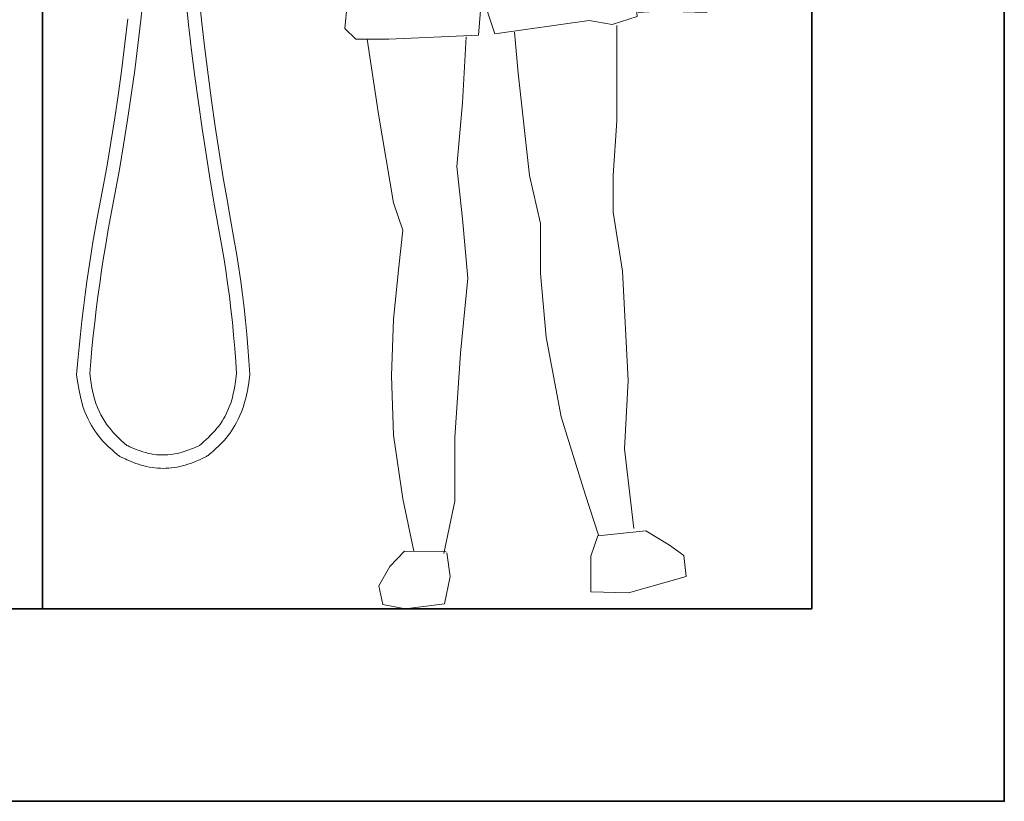
# Model space of a CAD drawing. Units: inches. Extents: x 64 to 1167, y 117 to 939.
# Tile 38 of 56: x 1121 to 1167, y 428 to 464. Entities that reach past the tile are written whole.
import ezdxf

# ---------------------------------------------------------------- set-up
doc = ezdxf.new("R2010")
doc.units = ezdxf.units.IN
doc.header["$MEASUREMENT"] = 0
for name, color, linetype, lineweight in [('A-ENTG', 8, 'Continuous', 18), ('A-FLOR-FIXT', 8, 'Continuous', 18), ('A-SECT', 7, 'Continuous', 35)]:
    doc.layers.add(name, color=color, linetype=linetype, lineweight=lineweight)

# ---------------------------------------------------------------- blocks, each defined once
blk = doc.blocks.new('A$C43851DCA')
at = {"linetype": 'ByBlock'}
for p, q in [((0.009394, 0.066918), (0.008245, 0.066783)), ((0.010881, 0.066467), (0.009394, 0.066918)), ((0.008245, 0.066783), (0.007206, 0.066287)), ((0.011698, 0.06601), (0.010881, 0.066467)), ((0.007206, 0.066287), (0.0065, 0.065469)), ((0.012995, 0.064742), (0.011698, 0.06601)), ((0.0065, 0.065469), (0.005873, 0.063886)), ((0.013812, 0.064066), (0.012995, 0.064742)), ((0.014181, 0.063564), (0.013812, 0.064066)), ((0.005873, 0.063886), (0.005683, 0.062753)), ((0.013627, 0.063023), (0.014107, 0.063203)), ((0.014107, 0.063203), (0.014181, 0.063564)), ((0.005683, 0.062753), (0.005535, 0.061845)), ((0.009658, 0.062341), (0.010064, 0.062753)), ((0.010064, 0.062753), (0.01047, 0.062843)), ((0.01047, 0.062843), (0.010807, 0.062708)), ((0.010807, 0.062708), (0.010844, 0.062566)), ((0.012215, 0.062115), (0.012995, 0.062798)), ((0.012995, 0.062798), (0.013627, 0.063023)), ((0.01359, 0.062978), (0.013179, 0.061298)), ((0.009658, 0.061755), (0.009658, 0.062341)), ((0.005535, 0.061845), (0.005461, 0.060802)), ((0.009953, 0.061163), (0.009658, 0.061755)), ((0.011882, 0.061343), (0.012215, 0.062115)), ((0.009732, 0.061343), (0.009173, 0.060757)), ((0.011846, 0.060712), (0.011882, 0.061343)), ((0.013179, 0.061298), (0.013069, 0.060757)), ((0.010322, 0.060757), (0.009953, 0.061163)), ((0.005461, 0.060802), (0.005683, 0.060397)), ((0.005683, 0.060397), (0.00602, 0.060165)), ((0.009173, 0.060757), (0.008393, 0.059804)), ((0.010543, 0.06021), (0.010322, 0.060757)), ((0.013069, 0.060757), (0.013253, 0.060442)), ((0.013253, 0.060442), (0.013364, 0.06003)), ((0.00602, 0.060165), (0.0065, 0.059624)), ((0.013364, 0.06003), (0.013179, 0.059624)), ((0.0065, 0.059624), (0.006721, 0.058807)), ((0.007728, 0.059534), (0.006911, 0.059444)), ((0.008393, 0.059804), (0.007728, 0.059534)), ((0.013179, 0.059624), (0.012552, 0.058897)), ((0.006721, 0.058807), (0.006948, 0.057674)), ((0.010844, 0.057764), (0.01047, 0.058897)), ((0.012552, 0.058897), (0.012215, 0.058446)), ((0.012215, 0.058446), (0.012067, 0.057905)), ((0.006948, 0.057674), (0.006948, 0.057313)), ((0.010733, 0.056772), (0.010623, 0.057809)), ((0.01125, 0.057538), (0.010844, 0.057764)), ((0.012067, 0.057905), (0.011882, 0.057538)), ((0.005999, 0.057487), (0.00523, 0.056785)), ((0.00689, 0.057326), (0.005999, 0.057487)), ((0.009953, 0.057017), (0.00689, 0.057326)), ((0.011882, 0.057538), (0.01125, 0.057538)), ((0.00523, 0.056785), (0.004086, 0.055614)), ((0.011355, 0.05647), (0.009953, 0.057017)), ((0.013269, 0.055614), (0.011355, 0.05647)), ((0.004086, 0.055614), (0.00185, 0.054133)), ((0.01397, 0.054912), (0.013269, 0.055614)), ((0.014223, 0.052266), (0.01397, 0.054912)), ((0.00185, 0.054133), (0.000828, 0.053199)), ((0.000828, 0.053199), (0.000511, 0.050476)), ((0.014292, 0.049929), (0.014223, 0.052266)), ((0.010654, 0.051642), (0.01097, 0.051172)), ((0.01097, 0.051172), (0.010781, 0.048294)), ((0.000511, 0.050476), (0.00019, 0.04915)), ((0.01416, 0.047122), (0.014292, 0.049929)), ((0.00019, 0.04915), (0, 0.047747)), ((0.002615, 0.048758), (0.002235, 0.047438)), ((0.010781, 0.048294), (0.011102, 0.046035)), ((0, 0.047747), (0.000258, 0.045726)), ((0.002235, 0.047438), (0.002552, 0.045256)), ((0.012378, 0.046582), (0.01378, 0.047045)), ((0.01378, 0.047045), (0.01416, 0.047122)), ((0.011102, 0.046035), (0.012378, 0.046582)), ((0.01397, 0.046891), (0.01416, 0.04541)), ((0.011545, 0.046112), (0.011419, 0.044863)), ((0.000258, 0.045726), (0.000448, 0.043775)), ((0.002552, 0.045256), (0.002936, 0.043151)), ((0.01416, 0.04541), (0.015119, 0.044863)), ((0.011419, 0.044863), (0.011419, 0.043775)), ((0.015119, 0.044863), (0.016522, 0.044084)), ((0.000448, 0.043775), (0.000638, 0.042449)), ((0.011419, 0.043775), (0.012056, 0.043228)), ((0.016522, 0.044084), (0.017349, 0.043389)), ((0.017349, 0.043389), (0.017924, 0.042217)), ((0.002936, 0.043151), (0.003063, 0.041284)), ((0.012056, 0.043228), (0.013522, 0.042842)), ((0.000638, 0.042449), (0.001276, 0.042217)), ((0.013522, 0.042842), (0.015309, 0.042449)), ((0.015309, 0.042449), (0.016458, 0.041515)), ((0.001276, 0.042217), (0.002936, 0.041438)), ((0.014929, 0.039726), (0.015119, 0.042294)), ((0.017924, 0.042217), (0.018435, 0.041129)), ((0.016458, 0.041515), (0.01697, 0.040736)), ((0.003063, 0.041284), (0.003253, 0.040035)), ((0.020871, 0.040711), (0.016163, 0.04046)), ((0.022052, 0.028454), (0.020871, 0.040711)), ((0.015135, 0.040151), (0.019901, 0.040209)), ((0.019901, 0.040209), (0.021335, 0.028512)), ((0.003253, 0.040035), (0.003379, 0.037775)), ((0.01397, 0.039494), (0.014929, 0.039726)), ((0.016316, 0.037395), (0.015082, 0.039713)), ((0.01174, 0.03887), (0.012441, 0.039333)), ((0.012441, 0.039333), (0.01397, 0.039494)), ((0.011034, 0.038631), (0.01174, 0.03887)), ((0.003891, 0.037074), (0.011034, 0.038631)), ((0.003379, 0.037775), (0.003891, 0.037074)), ((0.016775, 0.035709), (0.016316, 0.037395)), ((0.003917, 0.037022), (0.003253, 0.035458)), ((0.016927, 0.034453), (0.016775, 0.035709)), ((0.003253, 0.035458), (0.003147, 0.03352)), ((0.016775, 0.033018), (0.016927, 0.034453)), ((0.003147, 0.03352), (0.003147, 0.03164)), ((0.008424, 0.033456), (0.008377, 0.032329)), ((0.016674, 0.030707), (0.016775, 0.033018)), ((0.008377, 0.032329), (0.008683, 0.030765)), ((0.003147, 0.03164), (0.003305, 0.029954)), ((0.008683, 0.030765), (0.0095, 0.029452)), ((0.016927, 0.027701), (0.016674, 0.030707)), ((0.003305, 0.029954), (0.003353, 0.028267)), ((0.0095, 0.029452), (0.009964, 0.027829)), ((0.0095, 0.026825), (0.009658, 0.028705)), ((0.003353, 0.028267), (0.003253, 0.02714)), ((0.021335, 0.028512), (0.020154, 0.027887)), ((0.020565, 0.028138), (0.022052, 0.028454)), ((0.009964, 0.027829), (0.010269, 0.026889)), ((0.015752, 0.027327), (0.016927, 0.027701)), ((0.018003, 0.027952), (0.01698, 0.027887)), ((0.020154, 0.027887), (0.018003, 0.027952)), ((0.010269, 0.026889), (0.014676, 0.027514)), ((0.014676, 0.027514), (0.015752, 0.027327)), ((0.015984, 0.022814), (0.015984, 0.027282)), ((0.003253, 0.02714), (0.003764, 0.026638)), ((0.005303, 0.026638), (0.0095, 0.026825)), ((0.008751, 0.023664), (0.008925, 0.026748)), ((0.011192, 0.02696), (0.011366, 0.025048)), ((0.003764, 0.026638), (0.005303, 0.026638)), ((0.004302, 0.026645), (0.004829, 0.02313)), ((0.011366, 0.025048), (0.011888, 0.020259)), ((0.008487, 0.020684), (0.008751, 0.023664)), ((0.004829, 0.02313), (0.005525, 0.018978)), ((0.01581, 0.020259), (0.015984, 0.022814)), ((0.008751, 0.018237), (0.008487, 0.020684)), ((0.011888, 0.020259), (0.01241, 0.018025)), ((0.01581, 0.018553), (0.01581, 0.020259)), ((0.005525, 0.018978), (0.005962, 0.017703)), ((0.016247, 0.015785), (0.01581, 0.018553)), ((0.009009, 0.015469), (0.008751, 0.018237)), ((0.01241, 0.018025), (0.01241, 0.015682)), ((0.005962, 0.017703), (0.005783, 0.015997)), ((0.005783, 0.015997), (0.005525, 0.013551)), ((0.01241, 0.015682), (0.012673, 0.012701)), ((0.016506, 0.01068), (0.016247, 0.015785)), ((0.008661, 0.011954), (0.009009, 0.015469)), ((0.005525, 0.013551), (0.005435, 0.010892)), ((0.012673, 0.012701), (0.013369, 0.008974)), ((0.008403, 0.008015), (0.008661, 0.011954)), ((0.005435, 0.010892), (0.005525, 0.008124)), ((0.016332, 0.007487), (0.016506, 0.01068)), ((0.013369, 0.008974), (0.014502, 0.005356)), ((0.005525, 0.008124), (0.005962, 0.005144)), ((0.008403, 0.005034), (0.008403, 0.008015)), ((0.016769, 0.003759), (0.016332, 0.007487)), ((0.005962, 0.005144), (0.006484, 0.002697)), ((0.014502, 0.005356), (0.015114, 0.003438)), ((0.007876, 0.002588), (0.008403, 0.005034)), ((0.015093, 0.003412), (0.014766, 0.002459)), ((0.017333, 0.003644), (0.015093, 0.003412)), ((0.018435, 0.002974), (0.017333, 0.003644)), ((0.019115, 0.002498), (0.018435, 0.002974)), ((0.006036, 0.002697), (0.005356, 0.001983)), ((0.007987, 0.002659), (0.006036, 0.002697)), ((0.008182, 0.001506), (0.008018, 0.002614)), ((0.014766, 0.002459), (0.014766, 0.000792)), ((0.019215, 0.001506), (0.019115, 0.002498)), ((0.005356, 0.001983), (0.004839, 0.001069)), ((0.007918, 0.000238), (0.008182, 0.001506)), ((0.016522, 0.000753), (0.019215, 0.001506)), ((0.004839, 0.001069), (0.005034, 0.0002)), ((0.014766, 0.000792), (0.016522, 0.000753)), ((0.005034, 0.0002), (0.006073, 0)), ((0.006073, 0), (0.007918, 0.000238))]:
    blk.add_line(p, q, dxfattribs=at)

msp = doc.modelspace()

# ---------------------------------------------------------------- linework, layer by layer
at = {"layer": 'A-FLOR-FIXT'}
for p, q in [((1126.404, 464.201), (1126.528, 465.37)), ((1128.515, 465.221), (1128.645, 464.002)), ((1129.26, 464.072), (1129.136, 465.244)), ((1125.667, 463.108), (1125.802, 464.269)), ((1126.268, 463.034), (1126.404, 464.201)), ((1128.645, 464.002), (1128.786, 462.785)), ((1129.4, 462.861), (1129.26, 464.072)), ((1125.519, 461.949), (1125.667, 463.108)), ((1126.12, 461.868), (1126.268, 463.034)), ((1128.786, 462.785), (1128.938, 461.57)), ((1129.552, 461.651), (1129.4, 462.861)), ((1125.36, 460.791), (1125.519, 461.949)), ((1125.96, 460.704), (1126.12, 461.868)), ((1128.938, 461.57), (1129.101, 460.356)), ((1129.714, 460.443), (1129.552, 461.651)), ((1125.189, 459.636), (1125.36, 460.791)), ((1125.788, 459.542), (1125.96, 460.704)), ((1129.101, 460.356), (1129.275, 459.144)), ((1129.887, 459.237), (1129.714, 460.443)), ((1125.006, 458.483), (1125.189, 459.636)), ((1125.604, 458.383), (1125.788, 459.542)), ((1129.275, 459.144), (1129.46, 457.935)), ((1130.071, 458.033), (1129.887, 459.237)), ((1124.811, 457.332), (1125.006, 458.483)), ((1125.407, 457.226), (1125.604, 458.383)), ((1130.266, 456.831), (1130.071, 458.033)), ((1129.46, 457.935), (1129.656, 456.727)), ((1124.603, 456.184), (1124.811, 457.332)), ((1125.199, 456.072), (1125.407, 457.226)), ((1129.656, 456.727), (1129.863, 455.521)), ((1130.472, 455.631), (1130.266, 456.831)), ((1124.384, 455.037), (1124.603, 456.184)), ((1124.98, 454.924), (1125.199, 456.072)), ((1130.188, 453.716), (1129.863, 455.521)), ((1130.558, 455.155), (1130.472, 455.631)), ((1124.273, 454.428), (1124.384, 455.034)), ((1124.87, 454.32), (1124.98, 454.924)), ((1130.797, 453.824), (1130.558, 455.155)), ((1124.168, 453.819), (1124.273, 454.428)), ((1124.765, 453.717), (1124.87, 454.32)), ((1130.9, 453.214), (1130.797, 453.824)), ((1124.068, 453.209), (1124.168, 453.819)), ((1124.666, 453.112), (1124.765, 453.717)), ((1130.188, 453.716), (1130.289, 453.113)), ((1123.973, 452.597), (1124.068, 453.209)), ((1124.572, 452.506), (1124.666, 453.112)), ((1130.289, 453.113), (1130.383, 452.508)), ((1130.995, 452.602), (1130.9, 453.214)), ((1123.884, 451.985), (1123.973, 452.597)), ((1124.484, 451.899), (1124.572, 452.506)), ((1130.383, 452.508), (1130.471, 451.903)), ((1131.084, 451.989), (1130.995, 452.602)), ((1123.8, 451.372), (1123.884, 451.985)), ((1131.165, 451.375), (1131.084, 451.989)), ((1124.401, 451.291), (1124.484, 451.899)), ((1130.471, 451.903), (1130.552, 451.296)), ((1123.721, 450.758), (1123.8, 451.372)), ((1124.323, 450.683), (1124.401, 451.291)), ((1130.552, 451.296), (1130.625, 450.688)), ((1131.24, 450.76), (1131.165, 451.375)), ((1123.648, 450.143), (1123.721, 450.758)), ((1124.251, 450.073), (1124.323, 450.683)), ((1130.625, 450.688), (1130.692, 450.078)), ((1131.308, 450.144), (1131.24, 450.76)), ((1123.581, 449.528), (1123.648, 450.143)), ((1131.368, 449.527), (1131.308, 450.144)), ((1124.184, 449.463), (1124.251, 450.073)), ((1130.692, 450.078), (1130.752, 449.469)), ((1123.519, 448.911), (1123.581, 449.528)), ((1124.122, 448.852), (1124.184, 449.463)), ((1130.752, 449.469), (1130.805, 448.858)), ((1131.422, 448.909), (1131.368, 449.527)), ((1123.462, 448.295), (1123.519, 448.911)), ((1124.066, 448.241), (1124.122, 448.852)), ((1130.805, 448.858), (1130.851, 448.246)), ((1131.469, 448.29), (1131.422, 448.909)), ((1123.462, 448.295), (1123.405, 447.616)), ((1124.02, 447.69), (1124.066, 448.241)), ((1130.851, 448.246), (1130.889, 447.662)), ((1131.51, 447.644), (1131.469, 448.29))]:
    msp.add_line(p, q, dxfattribs=at)
for points in [[(1123.405, 447.616), (1123.458, 447.226), (1123.516, 446.884), (1123.579, 446.585), (1123.647, 446.325), (1123.717, 446.096), (1123.791, 445.895), (1123.866, 445.715), (1123.943, 445.551), (1124.021, 445.399), (1124.099, 445.256), (1124.179, 445.122), (1124.26, 444.997), (1124.343, 444.878), (1124.428, 444.765), (1124.516, 444.658), (1124.606, 444.554), (1124.699, 444.455), (1124.792, 444.36), (1124.885, 444.269), (1124.976, 444.185), (1125.061, 444.108), (1125.141, 444.039), (1125.211, 443.979), (1125.271, 443.928), (1125.32, 443.888), (1125.36, 443.856), (1125.394, 443.831), (1125.426, 443.809), (1125.459, 443.79), (1125.496, 443.771), (1125.542, 443.749), (1125.598, 443.723), (1125.668, 443.691), (1125.752, 443.653), (1125.846, 443.612), (1125.95, 443.568), (1126.061, 443.524), (1126.179, 443.479), (1126.301, 443.437), (1126.426, 443.397), (1126.552, 443.362), (1126.68, 443.332), (1126.808, 443.306), (1126.936, 443.285), (1127.066, 443.269), (1127.196, 443.257), (1127.326, 443.25), (1127.456, 443.247), (1127.586, 443.25), (1127.716, 443.257), (1127.846, 443.269), (1127.975, 443.285), (1128.104, 443.306), (1128.232, 443.332), (1128.36, 443.362), (1128.486, 443.397), (1128.611, 443.437), (1128.733, 443.479), (1128.851, 443.524), (1128.962, 443.568), (1129.066, 443.612), (1129.16, 443.653), (1129.243, 443.691), (1129.314, 443.723), (1129.37, 443.749), (1129.415, 443.771), (1129.453, 443.79), (1129.486, 443.809), (1129.518, 443.831), (1129.552, 443.856), (1129.592, 443.888), (1129.641, 443.928), (1129.701, 443.979), (1129.771, 444.039), (1129.85, 444.108), (1129.936, 444.185), (1130.026, 444.269), (1130.12, 444.36), (1130.213, 444.455), (1130.306, 444.554), (1130.396, 444.658), (1130.484, 444.765), (1130.569, 444.878), (1130.652, 444.997), (1130.733, 445.122), (1130.812, 445.256), (1130.891, 445.399), (1130.969, 445.551), (1131.045, 445.715), (1131.121, 445.895), (1131.195, 446.098), (1131.266, 446.328), (1131.333, 446.592), (1131.397, 446.896), (1131.456, 447.245), (1131.51, 447.644)], [(1125.76, 444.319), (1125.511, 444.537), (1125.3, 444.739), (1125.12, 444.927), (1124.967, 445.104), (1124.838, 445.273), (1124.727, 445.436), (1124.63, 445.597), (1124.542, 445.758), (1124.46, 445.923), (1124.383, 446.097), (1124.31, 446.286), (1124.243, 446.498), (1124.18, 446.738), (1124.122, 447.012), (1124.068, 447.328), (1124.02, 447.69)], [(1130.889, 447.662), (1130.841, 447.309), (1130.789, 447.001), (1130.734, 446.734), (1130.675, 446.503), (1130.613, 446.301), (1130.548, 446.124), (1130.483, 445.967), (1130.416, 445.824), (1130.348, 445.692), (1130.279, 445.567), (1130.208, 445.449), (1130.133, 445.336), (1130.054, 445.227), (1129.969, 445.12), (1129.879, 445.014), (1129.781, 444.908), (1129.676, 444.8), (1129.568, 444.695), (1129.462, 444.596), (1129.364, 444.506), (1129.278, 444.429), (1129.21, 444.369), (1129.164, 444.329), (1129.146, 444.314)], [(1129.152, 444.319), (1128.868, 444.195), (1128.614, 444.096), (1128.386, 444.02), (1128.181, 443.964), (1127.997, 443.924), (1127.829, 443.898), (1127.675, 443.883), (1127.531, 443.876), (1127.394, 443.874), (1127.263, 443.878), (1127.136, 443.887), (1127.011, 443.902), (1126.888, 443.923), (1126.764, 443.95), (1126.638, 443.982), (1126.509, 444.022), (1126.377, 444.067), (1126.244, 444.116), (1126.117, 444.166), (1125.999, 444.215), (1125.897, 444.259), (1125.813, 444.295), (1125.755, 444.321)]]:
    msp.add_lwpolyline(points, dxfattribs=at)
at = {"layer": 'A-SECT'}
for p, q in [((1157.813, 436.679), (1157.813, 556.679)), ((1121.813, 436.679), (1121.813, 540.679)), ((991.813, 436.679), (1157.813, 436.679))]:
    msp.add_line(p, q, dxfattribs=at)
msp.add_lwpolyline([(982.813, 427.679), (1166.813, 427.679), (1166.813, 565.679), (982.813, 565.679)], close=True, dxfattribs=at)

# ---------------------------------------------------------------- block references
at = {"layer": 'A-ENTG', "xscale": 1000, "yscale": 1000, "zscale": 1000}
msp.add_blockref('A$C43851DCA', (1132.705, 436.679), dxfattribs=at)

doc.saveas('drawing.dxf')
